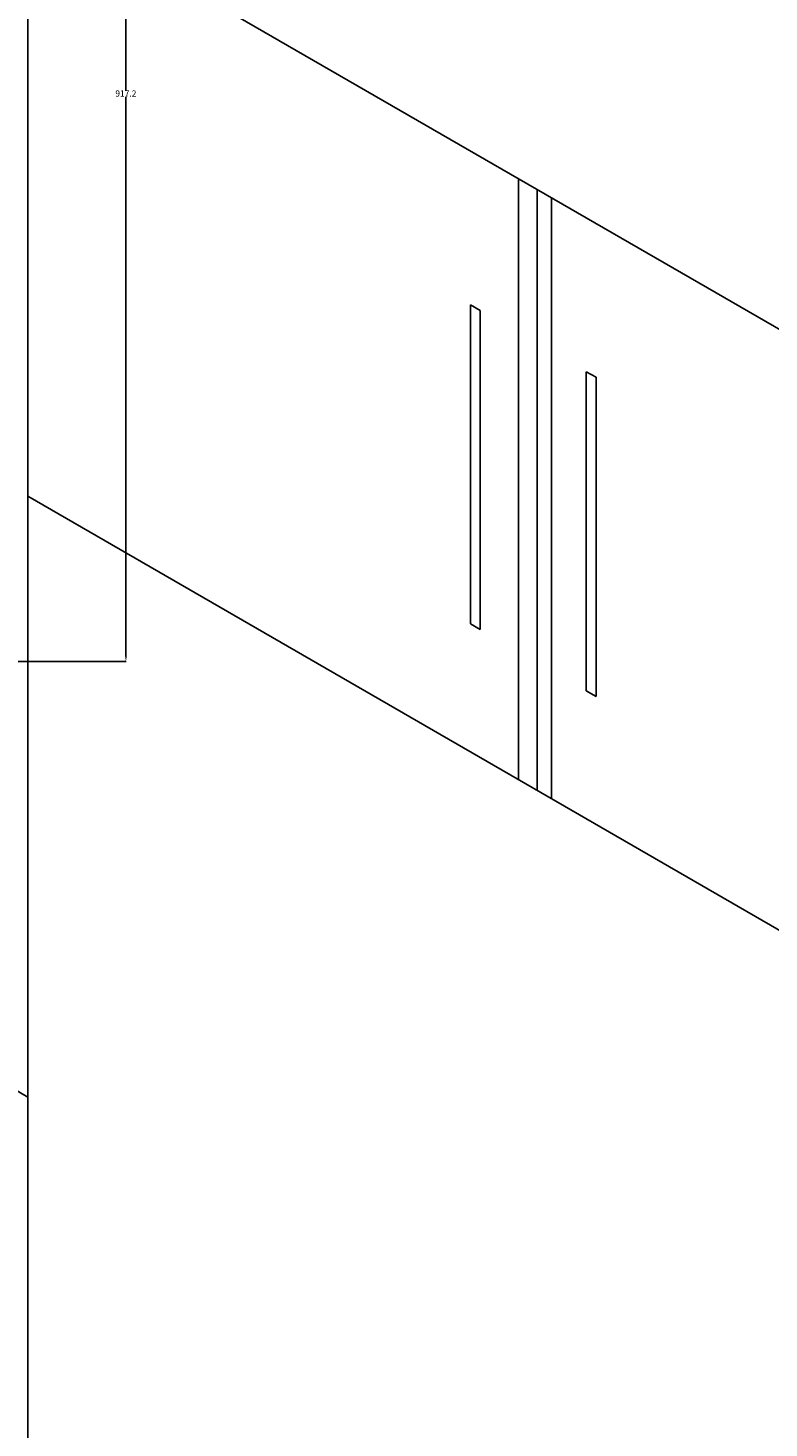
# Model space of a CAD drawing. Units: metres. Extents: x -2391 to 4922, y -635 to 4845.
# Tile 35 of 37: x 3149 to 3747, y 1238 to 2368. Entities that reach past the tile are written whole.
import ezdxf

# ---------------------------------------------------------------- set-up
doc = ezdxf.new("R2010")
doc.units = ezdxf.units.M
doc.header["$MEASUREMENT"] = 0
doc.layers.add('A-ANNO-DIMS', color=2, linetype='Continuous', lineweight=18)
doc.layers.add('A-FLOR-FIXT', color=3, linetype='Continuous', lineweight=25)
doc.styles.get("Standard").update_dxf_attribs({"font": 'arial.ttf'})
doc.dimstyles.get("Standard").update_dxf_attribs({"dimtxt": 5, "dimasz": 4, "dimexe": 0.18, "dimexo": 0.0625, "dimgap": 0.09, "dimtad": 0, "dimtih": 1, "dimtoh": 1, "dimdec": 0, "dimzin": 0, "dimdsep": 46, "dimtxsty": 'Standard', "dimcen": 0.09, "dimadec": 0, "dimazin": 0, "dimtfac": 1, "dimtdec": 0, "dimtofl": 0, "dimtmove": 0, "dimatfit": 3, "dimfxl": 1, "dimtolj": 1, "dimtzin": 0, "dimarcsym": 0})

# ---------------------------------------------------------------- blocks, each defined once
blk = doc.blocks.new('HANDLE-DOOR-262')
for p, q in [((0, 262.1), (0, 4.6)), ((0, 262.1), (7.9, 257.6)), ((7.9, 0), (7.9, 257.6)), ((0, 4.6), (7.9, 0))]:
    blk.add_line(p, q)
blk = doc.blocks.new('*D8')
at = {"layer": 'A-ANNO-DIMS', "color": 0, "lineweight": -2, "transparency": 16777216}
for p, q in [((-2047.3, 3005.2), (-2047.3, -631.4)), ((4577.8, 2350.2), (4577.8, -631.4)), ((-2043.3, -631.2), (1257.6, -631.2)), ((4573.8, -631.2), (1272.8, -631.2))]:
    blk.add_line(p, q, dxfattribs=at)
at = {"layer": 'A-ANNO-DIMS', "color": 0, "transparency": 16777216}
for points in [[(-2043.3, -630.6), (-2043.3, -631.9), (-2047.3, -631.2)], [(4573.8, -630.6), (4573.8, -631.9), (4577.8, -631.2)]]:
    blk.add_solid(points, dxfattribs=at)
at = {"layer": 'Defpoints', "color": 0, "transparency": 16777216}
for p in [(-2047.3, 3005.3), (4577.8, 2350.3), (4577.8, -631.2)]:
    blk.add_point(p, dxfattribs=at)
at = {"layer": 'A-ANNO-DIMS', "color": 0, "transparency": 16777216, "insert": (1265.2, -631.2), "char_height": 5, "attachment_point": 5}
blk.add_mtext('\\A1;6625', dxfattribs=at)
blk = doc.blocks.new('*D13')
at = {"layer": 'A-ANNO-DIMS', "color": 0, "lineweight": -2, "transparency": 16777216}
for p, q in [((2891.5, 2774), (3228.1, 2774)), ((3227.9, 2770), (3227.9, 2318)), ((3227.9, 1860.8), (3227.9, 2312.8)), ((2891.5, 1856.8), (3228.1, 1856.8))]:
    blk.add_line(p, q, dxfattribs=at)
at = {"layer": 'A-ANNO-DIMS', "color": 0, "transparency": 16777216}
for points in [[(3227.3, 2770), (3228.6, 2770), (3227.9, 2774)], [(3227.3, 1860.8), (3228.6, 1860.8), (3227.9, 1856.8)]]:
    blk.add_solid(points, dxfattribs=at)
at = {"layer": 'Defpoints', "color": 0, "transparency": 16777216}
for p in [(2891.4, 2774), (2891.4, 1856.8), (3227.9, 1856.8)]:
    blk.add_point(p, dxfattribs=at)
at = {"layer": 'A-ANNO-DIMS', "color": 0, "transparency": 16777216, "insert": (3227.9, 2315.4), "char_height": 5, "attachment_point": 5}
blk.add_mtext('\\A1;917.2', dxfattribs=at)
blk = doc.blocks.new('*D28')
at = {"layer": 'A-ANNO-DIMS', "color": 0, "lineweight": -2, "transparency": 16777216}
for p, q in [((3148.8, 2475.3), (3317.2, 2766.8)), ((3320.5, 2764.7), (3723.9, 2531.8)), ((4136.3, 2293.7), (3733, 2526.6)), ((3971.6, 2000.3), (4139.9, 2291.8))]:
    blk.add_line(p, q, dxfattribs=at)
at = {"layer": 'A-ANNO-DIMS', "color": 0, "transparency": 16777216}
for points in [[(3320.9, 2765.3), (3320.2, 2764.1), (3317.1, 2766.7)], [(4136.7, 2294.3), (4136, 2293.1), (4139.8, 2291.7)]]:
    blk.add_solid(points, dxfattribs=at)
at = {"layer": 'Defpoints', "color": 0, "transparency": 16777216}
for p in [(3148.8, 2475.3), (4139.8, 2291.7), (3971.5, 2000.3)]:
    blk.add_point(p, dxfattribs=at)
at = {"layer": 'A-ANNO-DIMS', "color": 0, "transparency": 16777216, "insert": (3728.4, 2529.2), "char_height": 5, "attachment_point": 5}
blk.add_mtext('\\A1;950', dxfattribs=at)

msp = doc.modelspace()

# ---------------------------------------------------------------- linework, layer by layer
at = {"layer": 'A-FLOR-FIXT'}
for p, q in [((550.7419, 3005.2763), (3148.8181, 1505.2763)), ((3148.8181, 2475.2763), (3148.8181, 1505.2763)), ((3148.8181, 2475.2763), (3971.5422, 2000.2763)), ((3545.1371, 2246.4614), (3545.1371, 1761.4614)), ((3560.1802, 1752.7763), (3560.1802, 2237.7763)), ((3571.6043, 2231.1805), (3571.6043, 1746.1805)), ((3148.8181, 1990.2763), (3971.5422, 1515.2763)), ((3148.8181, 1505.2763), (3148.8181, 625.2763))]:
    msp.add_line(p, q, dxfattribs=at)

# ---------------------------------------------------------------- block references
at = {"layer": 'A-FLOR-FIXT', "rotation": 180}
msp.add_blockref('HANDLE-DOOR-262', (3514.1805, 2144.8248), dxfattribs=at)
at = {"layer": 'A-FLOR-FIXT'}
msp.add_blockref('HANDLE-DOOR-262', (3599.804, 1828.688), dxfattribs=at)

# ---------------------------------------------------------------- dimensions: what is measured, and where the dimension line sits
at = {"layer": 'A-ANNO-DIMS'}
dim = msp.add_linear_dim(base=(4577.76, -631.2237), p1=(-2047.3343, 3005.2763), p2=(4577.76, 2350.2763), dimstyle='Standard', override={"dimdec": 0, "dimlfac": 1, "dimrnd": 0, "dimzin": 0, "dimdsep": 46, "dimlunit": 2}, dxfattribs=at)
dim.commit()
dim.dimension.update_dxf_attribs({"geometry": '*D8', "text_midpoint": (1265.2128, -631.2237)})
for base, p1, p2, angle, override, picture, middle in [((3227.9324, 1856.8211), (2891.4324, 2773.9801), (2891.4324, 1856.8211), 270, {"dimdec": 1, "dimlfac": 1, "dimrnd": 0, "dimzin": 0, "dimdsep": 46, "dimlunit": 2}, '*D13', (3227.9324, 2315.4006)), ((4139.7922, 2291.6938), (3148.8181, 2475.2763), (3971.5422, 2000.2763), 330, {"dimdec": 0, "dimlfac": 1, "dimrnd": 0, "dimzin": 0, "dimdsep": 46, "dimlunit": 2}, '*D28', (3728.4302, 2529.1938))]:
    dim = msp.add_linear_dim(base=base, p1=p1, p2=p2, angle=angle, dimstyle='Standard', override=override, dxfattribs=at)
    dim.commit()
    dim.dimension.update_dxf_attribs({"geometry": picture, "text_midpoint": middle})

doc.saveas('drawing.dxf')
